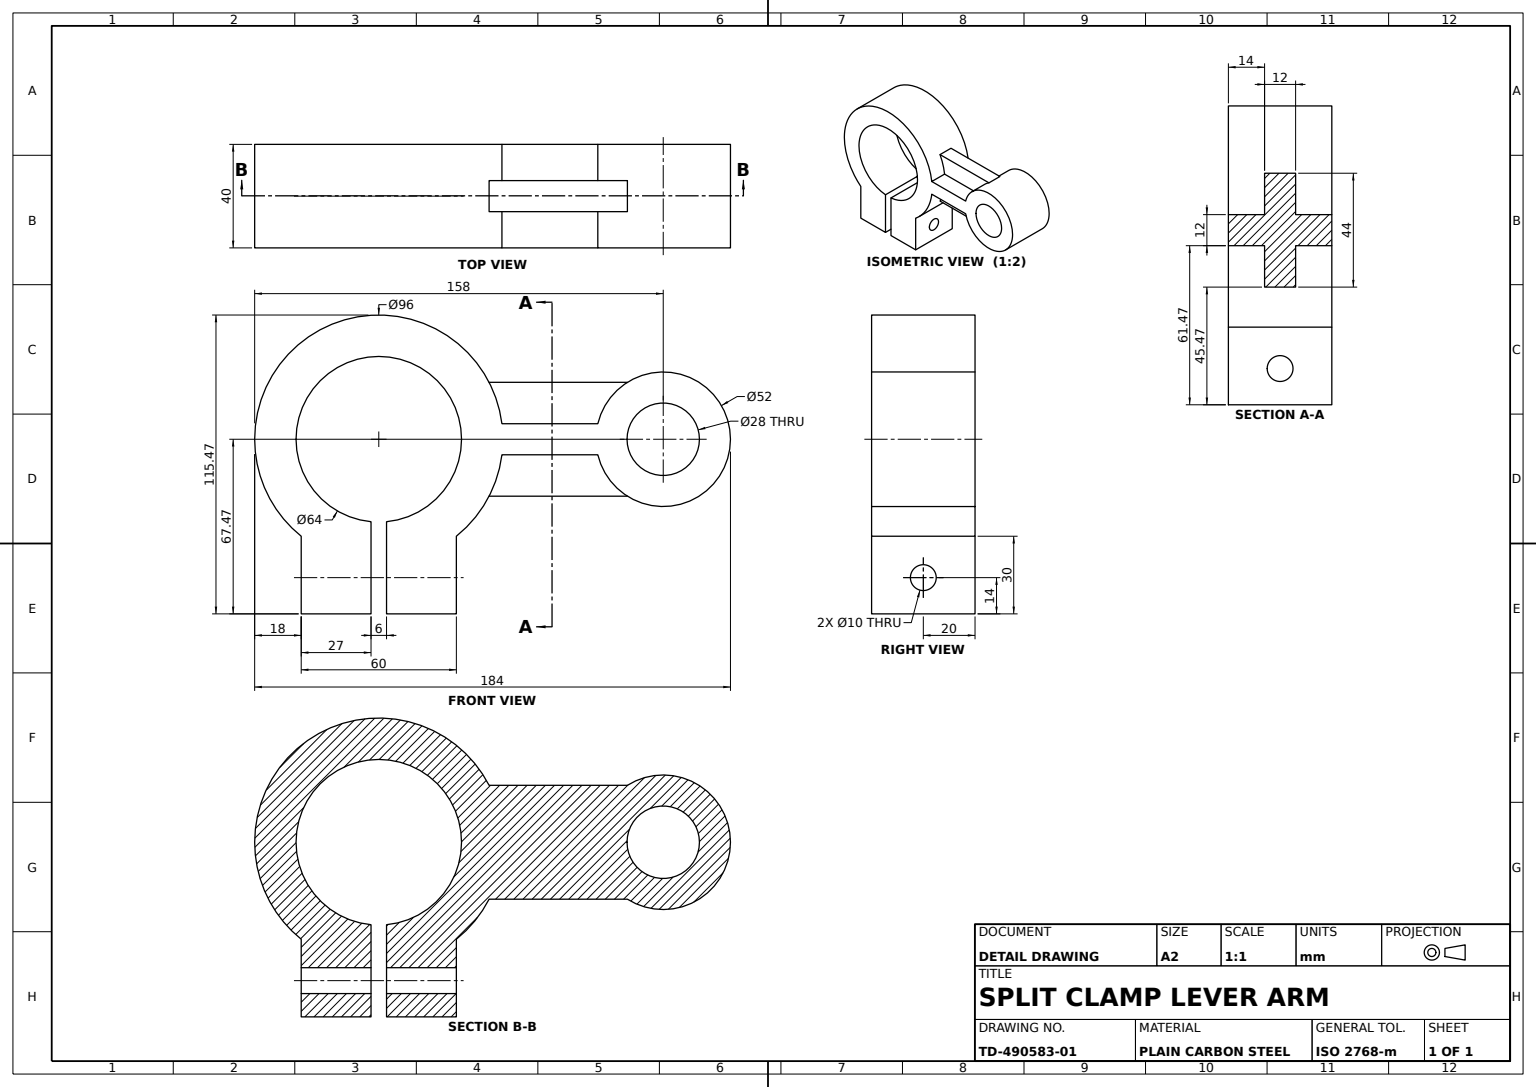
from build123d import *

# Parameters (mm, degrees)
CLAMP_RING_SKETCH_R             = 48
CLAMP_RING_96_DEPTH             = 40
CLAMP_START                     = -40
CLAMP_LUG_DEPTH                 = 40
CLAMP_BORE_AND_SPLIT_SLOT_DEPTH = 40
PIVOT_EYE_SKETCH_R              = 26
PIVOT_EYE_52_DEPTH              = 40
CONNECTING_START                = -40
CONNECTING_ARM_DEPTH            = 40
ARM_RIB_A_DEPTH                 = 16
ARM_RIB_B_DEPTH                 = 16
PIVOT_BORE_SKETCH_R             = 14
PIVOT_BORE_28_DEPTH             = 40
CLAMP_SCREW_HOLE_SKETCH_R       = 5
CLAMP_SCREW_HOLE_10_DEPTH       = 80


with BuildPart() as part:
    # Clamp Ring Sketch → Clamp Ring Ø96 (new body)
    with BuildSketch(Plane.XY):
        Circle(CLAMP_RING_SKETCH_R)
    extrude(amount=CLAMP_RING_96_DEPTH)

    # Clamp Lug Sketch → Clamp Lug (add)
    with BuildSketch(Plane.XY.offset(40).offset(CLAMP_START)):
        with BuildLine():
            Line((30, -67.46998799), (30, -37.46998799))
            ThreePointArc((30, -37.46998799), (0, -48), (-30, -37.46998799))
            Line((-30, -37.46998799), (-30, -67.46998799))
            Line((-30, -67.46998799), (30, -67.46998799))
        make_face()
    extrude(amount=CLAMP_LUG_DEPTH)

    # Clamp Bore and Split Sketch → Clamp Bore and Split Slot (cut)
    with BuildSketch(Plane.XY.offset(40)):
        with BuildLine():
            Line((-3, -67.46998799), (3, -67.46998799))
            Line((3, -67.46998799), (3, -31.859064644))
            ThreePointArc((3, -31.859064644), (0, 32), (-3, -31.859064644))
            Line((-3, -31.859064644), (-3, -67.46998799))
        make_face()
    extrude(amount=-CLAMP_BORE_AND_SPLIT_SLOT_DEPTH, mode=Mode.SUBTRACT)



with BuildPart() as body_2:
    # Pivot Eye Sketch → Pivot Eye Ø52 (new body)
    with BuildSketch(Plane.XY.offset(40)):
        with Locations((110, 0)):
            Circle(PIVOT_EYE_SKETCH_R)
    extrude(amount=-PIVOT_EYE_52_DEPTH)


with BuildPart() as part_1:
    add(part.part)

    add(body_2.part)  # Connecting Arm merges body 2
    # Connecting Arm Sketch → Connecting Arm (add)
    with BuildSketch(Plane.XY.offset(40).offset(CONNECTING_START)):
        with BuildLine():
            Line((47.623523599, 6), (84.701778719, 6))
            ThreePointArc((84.701778719, 6), (84, 0), (84.701778719, -6))
            Line((84.701778719, -6), (47.623523599, -6))
            ThreePointArc((47.623523599, -6), (48, 0), (47.623523599, 6))
        make_face()
    extrude(amount=CONNECTING_ARM_DEPTH)

    # Arm Rib A Sketch → Arm Rib A (add)
    with BuildSketch(Plane(origin=(0, 6, 0), x_dir=(1, 0, 0), z_dir=(0, 1, 0))):
        Polygon((98.516804154, -14), (110.350889359, -14), (110.350889359, -26), (98.516804154, -26), (39.268352847, -26), (39.268352847, -20), (39.268352847, -14), align=None)
    extrude(amount=ARM_RIB_A_DEPTH)

    # Arm Rib B Sketch → Arm Rib B (add)
    with BuildSketch(Plane.XZ.offset(6)):
        Polygon((38.239733901, 20), (38.239733901, 26), (110.350889359, 26), (110.350889359, 14), (38.239733901, 14), align=None)
    extrude(amount=ARM_RIB_B_DEPTH)

    # Pivot Bore Sketch → Pivot Bore Ø28 (cut)
    with BuildSketch(Plane.XY.offset(40)):
        with Locations((110, 0)):
            Circle(PIVOT_BORE_SKETCH_R)
    extrude(amount=-PIVOT_BORE_28_DEPTH, mode=Mode.SUBTRACT)

    # Clamp Screw Hole Sketch → Clamp Screw Hole Ø10 (cut)
    with BuildSketch(Plane(origin=(30, 0, 0), x_dir=(0, 0, -1), z_dir=(1, 0, 0))):
        with Locations(Location((-20, -53.46998799, 0), (0, 0, 270))):
            Circle(CLAMP_SCREW_HOLE_SKETCH_R)
    extrude(amount=-CLAMP_SCREW_HOLE_10_DEPTH, mode=Mode.SUBTRACT)


solid = part_1.part
